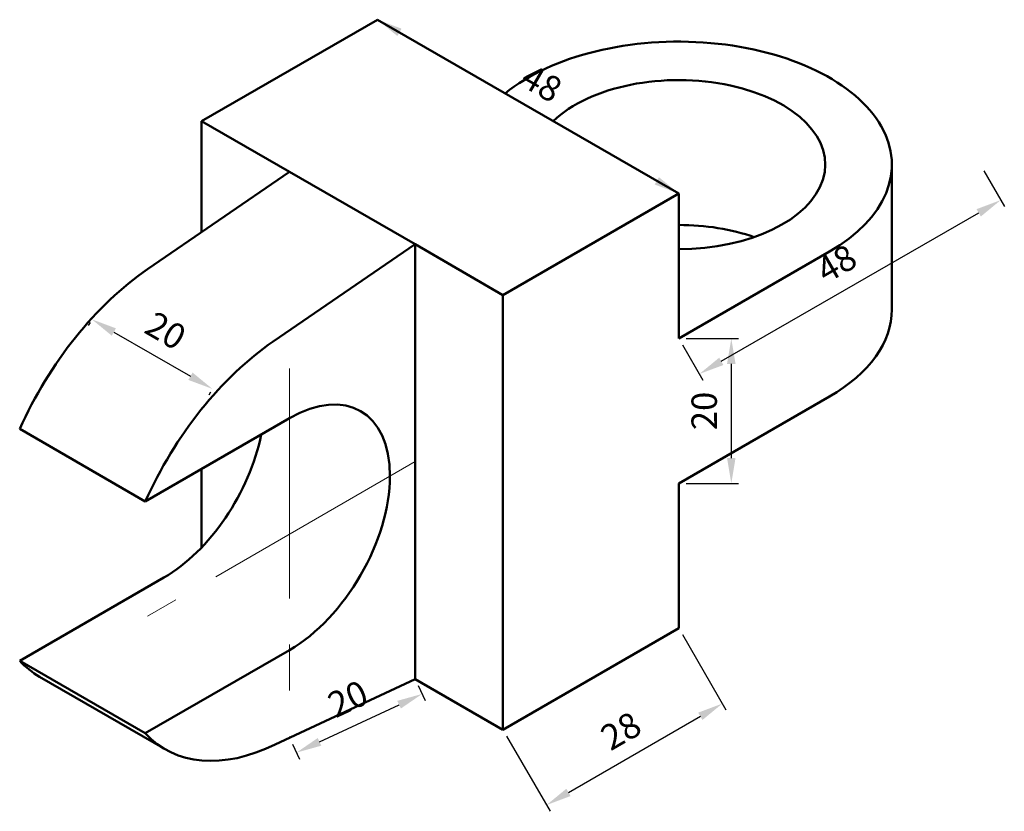
# Model space of a CAD drawing. Units: millimetres. Extents: x 2870 to 3006, y 794 to 903.
import ezdxf

# ---------------------------------------------------------------- set-up
doc = ezdxf.new("R2010")
doc.units = ezdxf.units.MM
doc.linetypes.add('CENTER', pattern=[50.8, 31.75, -6.35, 6.35, -6.35])
for name, color, linetype, lineweight in [('M-CNTR', 1, 'CENTER', 18), ('M-DIMS', 3, 'Continuous', 25), ('M-OUTL', 7, 'Continuous', 50)]:
    doc.layers.add(name, color=color, linetype=linetype, lineweight=lineweight)
doc.styles.get("Standard").update_dxf_attribs({"font": 'arial.ttf'})
doc.dimstyles.new('AM_ISO$0', dxfattribs={"dimtxt": 3.5, "dimasz": 3.5, "dimexe": 1, "dimexo": 1, "dimgap": 1.5, "dimtad": 1, "dimdsep": 46, "dimtxsty": 'Standard', "dimcen": 0, "dimclrd": 256, "dimclre": 256, "dimclrt": 2, "dimadec": 0, "dimazin": 2, "dimtp": 0.1, "dimtm": 0.1, "dimtfac": 0.71, "dimtdec": 3, "dimtmove": 0, "dimatfit": 3, "dimfxl": 1, "dimlwd": -1, "dimlwe": -1, "dimarcsym": 1})

# ---------------------------------------------------------------- blocks, each defined once
blk = doc.blocks.new('*D3')
at = {"layer": 'Defpoints', "color": 0, "transparency": 16777216}
for p in [(2880.21, 861.86), (2896.59, 851.83), (2896.84, 852.26)]:
    blk.add_point(p, dxfattribs=at)
at = {"layer": 'M-DIMS', "color": 0, "linetype": 'ByBlock', "transparency": 16777216}
for p, q in [((2879.71, 860.99), (2879.46, 860.56)), ((2882.99, 859.68), (2893.56, 853.58)), ((2896.34, 851.39), (2896.09, 850.96))]:
    blk.add_line(p, q, dxfattribs=at)
at = {"layer": 'M-DIMS', "color": 0, "transparency": 16777216}
for points in [[(2883.28, 860.19), (2882.7, 859.18), (2879.96, 861.43)], [(2893.85, 854.08), (2893.27, 853.07), (2896.59, 851.83)]]:
    blk.add_solid(points, dxfattribs=at)
at = {"layer": 'M-DIMS', "color": 0, "transparency": 16777216, "insert": (2889.92, 859.48), "char_height": 3.5, "attachment_point": 5, "rotation": 330}
blk.add_mtext('20', dxfattribs=at)
blk = doc.blocks.new('*D4')
at = {"layer": 'Defpoints', "color": 0, "transparency": 16777216}
for p in [(2919.35, 902.79), (2960.92, 878.79), (2960.92, 878.79)]:
    blk.add_point(p, dxfattribs=at)
at = {"layer": 'M-DIMS', "color": 0, "linetype": 'ByBlock', "transparency": 16777216}
blk.add_line((2922.38, 901.04), (2957.89, 880.54), dxfattribs=at)
at = {"layer": 'M-DIMS', "color": 0, "transparency": 16777216}
for points in [[(2922.67, 901.55), (2922.09, 900.54), (2919.35, 902.79)], [(2958.18, 881.05), (2957.59, 880.04), (2960.92, 878.79)]]:
    blk.add_solid(points, dxfattribs=at)
at = {"layer": 'M-DIMS', "color": 0, "transparency": 16777216, "insert": (2941.78, 893.64), "char_height": 3.5, "attachment_point": 5, "rotation": 330}
blk.add_mtext('48', dxfattribs=at)
blk = doc.blocks.new('*D5')
at = {"layer": 'Defpoints', "color": 0, "transparency": 16777216}
for p in [(2960.92, 818.79), (2966.92, 808.4), (2936.67, 804.79)]:
    blk.add_point(p, dxfattribs=at)
at = {"layer": 'M-DIMS', "color": 0, "linetype": 'ByBlock', "transparency": 16777216}
for p, q in [((2961.42, 817.92), (2967.42, 807.53)), ((2945.7, 796.15), (2963.89, 806.65)), ((2937.17, 803.92), (2943.17, 793.53))]:
    blk.add_line(p, q, dxfattribs=at)
at = {"layer": 'M-DIMS', "color": 0, "transparency": 16777216}
for points in [[(2963.59, 807.15), (2964.18, 806.14), (2966.92, 808.4)], [(2945.41, 796.65), (2945.99, 795.64), (2942.67, 794.4)]]:
    blk.add_solid(points, dxfattribs=at)
at = {"layer": 'M-DIMS', "color": 0, "transparency": 16777216, "insert": (2953.15, 804.24), "char_height": 3.5, "attachment_point": 5, "rotation": 30}
blk.add_mtext('28', dxfattribs=at)
blk = doc.blocks.new('*D6')
at = {"layer": 'Defpoints', "color": 0, "transparency": 16777216}
for p in [(2924.54, 811.79), (2925.51, 809.73), (2907.22, 803.7)]:
    blk.add_point(p, dxfattribs=at)
at = {"layer": 'M-DIMS', "color": 0, "linetype": 'ByBlock', "transparency": 16777216}
for p, q in [((2924.97, 810.88), (2925.93, 808.82)), ((2911.36, 803.12), (2922.34, 808.25)), ((2907.65, 802.79), (2908.61, 800.73))]:
    blk.add_line(p, q, dxfattribs=at)
at = {"layer": 'M-DIMS', "color": 0, "transparency": 16777216}
for points in [[(2922.09, 808.78), (2922.58, 807.72), (2925.51, 809.73)], [(2911.11, 803.65), (2911.6, 802.59), (2908.19, 801.64)]]:
    blk.add_solid(points, dxfattribs=at)
at = {"layer": 'M-DIMS', "color": 0, "transparency": 16777216, "insert": (2915.45, 808.66), "char_height": 3.5, "attachment_point": 5, "rotation": 25.0419}
blk.add_mtext('20', dxfattribs=at)
blk = doc.blocks.new('*D7')
at = {"layer": 'Defpoints', "color": 0, "transparency": 16777216}
for p in [(2960.92, 858.79), (2960.92, 838.79), (2968.16, 838.79)]:
    blk.add_point(p, dxfattribs=at)
at = {"layer": 'M-DIMS', "color": 0, "linetype": 'ByBlock', "transparency": 16777216}
for p, q in [((2961.92, 858.79), (2969.16, 858.79)), ((2968.16, 855.29), (2968.16, 842.29)), ((2961.92, 838.79), (2969.16, 838.79))]:
    blk.add_line(p, q, dxfattribs=at)
at = {"layer": 'M-DIMS', "color": 0, "transparency": 16777216}
for points in [[(2967.57, 855.29), (2968.74, 855.29), (2968.16, 858.79)], [(2967.57, 842.29), (2968.74, 842.29), (2968.16, 838.79)]]:
    blk.add_solid(points, dxfattribs=at)
at = {"layer": 'M-DIMS', "color": 0, "transparency": 16777216, "insert": (2964.87, 848.79), "char_height": 3.5, "attachment_point": 5, "rotation": 90}
blk.add_mtext('20', dxfattribs=at)
blk = doc.blocks.new('*D8')
at = {"layer": 'Defpoints', "color": 0, "transparency": 16777216}
for p in [(3002.49, 882.79), (3005.32, 877.89), (2960.92, 858.79)]:
    blk.add_point(p, dxfattribs=at)
at = {"layer": 'M-DIMS', "color": 0, "linetype": 'ByBlock', "transparency": 16777216}
for p, q in [((3002.99, 881.92), (3005.82, 877.02)), ((2966.78, 855.64), (3002.28, 876.14)), ((2961.42, 857.92), (2964.25, 853.02))]:
    blk.add_line(p, q, dxfattribs=at)
at = {"layer": 'M-DIMS', "color": 0, "transparency": 16777216}
for points in [[(3001.99, 876.64), (3002.58, 875.63), (3005.32, 877.89)], [(2966.49, 856.14), (2967.07, 855.13), (2963.75, 853.89)]]:
    blk.add_solid(points, dxfattribs=at)
at = {"layer": 'M-DIMS', "color": 0, "transparency": 16777216, "insert": (2982.89, 868.74), "char_height": 3.5, "attachment_point": 5, "rotation": 30}
blk.add_mtext('48', dxfattribs=at)

msp = doc.modelspace()

# ---------------------------------------------------------------- linework, layer by layer
at = {"layer": 'M-CNTR'}
for p, q in [((2907.223, 854.662), (2907.223, 803.698)), ((2924.543, 841.79), (2887.619, 820.472))]:
    msp.add_line(p, q, dxfattribs=at)
at = {"layer": 'M-OUTL'}
for p, q in [((2919.347, 902.79), (2895.098, 888.79)), ((2960.916, 878.79), (2919.347, 902.79)), ((2895.098, 888.79), (2907.223, 881.79)), ((2895.098, 888.79), (2895.098, 873.476)), ((2907.223, 881.79), (2887.636, 868.36)), ((2924.543, 871.79), (2907.223, 881.79)), ((2990.305, 882.488), (2990.31, 862.79)), ((2960.916, 878.79), (2936.667, 864.79)), ((2960.916, 858.79), (2960.916, 878.79)), ((2924.543, 871.79), (2904.957, 858.36)), ((2936.667, 864.79), (2924.543, 871.79)), ((2924.543, 871.79), (2924.543, 811.79)), ((2924.543, 871.79), (2936.667, 864.79)), ((2981.701, 870.79), (2960.916, 858.79)), ((2936.667, 864.79), (2936.667, 804.79)), ((2960.916, 838.79), (2981.701, 850.79)), ((2907.223, 847.79), (2887.323, 836.301)), ((2870.002, 846.301), (2887.323, 836.301)), ((2895.098, 829.958), (2895.098, 840.79)), ((2960.916, 818.79), (2960.916, 838.79)), ((2889.902, 825.79), (2870.002, 814.301)), ((2936.667, 804.79), (2960.916, 818.79)), ((2907.223, 815.79), (2887.323, 804.301)), ((2870.002, 814.301), (2887.323, 804.301)), ((2872.756, 812.092), (2890.076, 802.092)), ((2905.26, 802.749), (2924.543, 811.79)), ((2924.543, 811.79), (2936.667, 804.79))]:
    msp.add_line(p, q, dxfattribs=at)
for centre, major_axis, start_param, end_param in [((2960.916, 882.79), (-29.394, 0), 2.3561945, 5.6652352), ((2960.916, 882.79), (-20.208, 0), 1.5707963, 5.742651), ((2960.916, 862.79), (-20.208, 0), 4.1712046, 4.712389), ((2889.902, 841.79), (-17.146, -29.698), 4.020565, 4.8895416), ((2960.916, 862.79), (-29.394, 0), 2.3561945, 3.1417291), ((2907.223, 831.79), (-17.146, -29.698), 4.020565, 4.8895416), ((2907.223, 831.79), (-9.798, -16.971), 7.0685835, 10.2101761), ((2889.902, 841.79), (-9.798, -16.971), 7.0685835, 8.3866995), ((2889.903, 841.791), (-17.147, -29.699), 6.1060353, 6.2831853), ((2907.223, 831.79), (-17.146, -29.698), 6.1060327, 6.987575)]:
    msp.add_ellipse(centre, major_axis=major_axis, ratio=0.5773503, start_param=start_param, end_param=end_param, dxfattribs=at)

# ---------------------------------------------------------------- dimensions: what is measured, and where the dimension line sits
at = {"layer": 'M-DIMS'}
for p1, p2, distance, override, picture, middle in [((2919.347, 902.79), (2960.916, 878.79), 0, {"dimclrd": 0, "dimclre": 0, "dimclrt": 0}, '*D4', (2941.775, 893.637)), ((2960.916, 858.79), (3002.485, 882.79), -5.66, {"dimpost": '', "dimclrd": 0, "dimclre": 0, "dimclrt": 0}, '*D8', (2982.887, 868.735)), ((2960.916, 858.79), (2960.916, 838.79), 7.241, {"dimpost": '', "dimclrd": 0, "dimclre": 0, "dimclrt": 0}, '*D7', (2964.871, 848.79)), ((2936.667, 804.79), (2960.916, 818.79), -12, {"dimclrd": 0, "dimclre": 0, "dimclrt": 0}, '*D5', (2953.148, 804.245))]:
    dim = msp.add_aligned_dim(p1=p1, p2=p2, distance=distance, dimstyle='AM_ISO$0', override=override, dxfattribs=at)
    dim.commit()
    dim.dimension.update_dxf_attribs({"geometry": picture, "text_midpoint": middle})
for p1, p2, distance, picture, middle in [((2880.209, 861.86), (2896.842, 852.257), -0.496, '*D3', (2889.921, 859.476)), ((2907.223, 803.698), (2924.543, 811.79), -2.276, '*D6', (2915.455, 808.66))]:
    dim = msp.add_aligned_dim(p1=p1, p2=p2, distance=distance, text='20', dimstyle='AM_ISO$0', override={"dimpost": '', "dimclrd": 0, "dimclre": 0, "dimclrt": 0}, dxfattribs=at)
    dim.commit()
    dim.dimension.update_dxf_attribs({"geometry": picture, "text_midpoint": middle})

doc.saveas('drawing.dxf')
